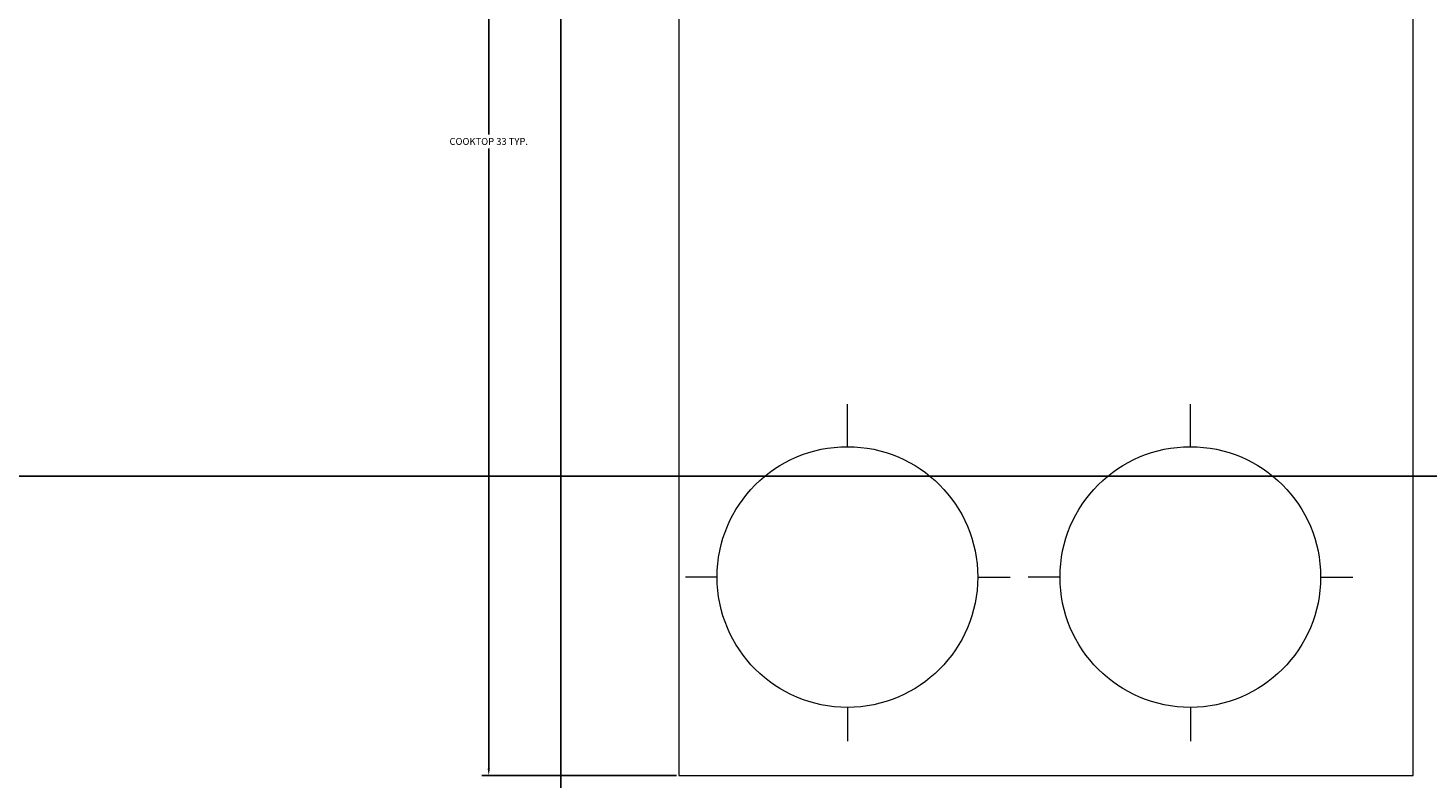
# Model space of a CAD drawing. Units: inches. Extents: x 1998 to 2588, y 1139 to 1977.
# Tile 22 of 134: x 2184 to 2220, y 1629 to 1648. Entities that reach past the tile are written whole.
import ezdxf

# ---------------------------------------------------------------- set-up
doc = ezdxf.new("R2010")
doc.units = ezdxf.units.IN
for name, color, linetype, lineweight in [('A-ANNO-DIMS', 2, 'Continuous', 18), ('A-EQPM', 21, 'Continuous', 18), ('A-FLOR-CASE', 32, 'Continuous', 25)]:
    doc.layers.add(name, color=color, linetype=linetype, lineweight=lineweight)
doc.styles.get("Standard").update_dxf_attribs({"font": 'arial.ttf'})
doc.dimstyles.get("Standard").update_dxf_attribs({"dimtxt": 0.18, "dimasz": 0.18, "dimexe": 0.18, "dimexo": 0.0625, "dimgap": 0.09, "dimtad": 0, "dimtih": 1, "dimtoh": 1, "dimdec": 4, "dimzin": 0, "dimdsep": 46, "dimtxsty": 'Standard', "dimcen": 0.09, "dimadec": 0, "dimazin": 0, "dimtfac": 1, "dimtdec": 4, "dimtofl": 0, "dimtmove": 0, "dimatfit": 3, "dimfxl": 1, "dimtolj": 1, "dimtzin": 0, "dimarcsym": 0})

# ---------------------------------------------------------------- blocks, each defined once
blk = doc.blocks.new('COOKTOP-FOUR-BURNER')
for p, q in [((13.348, 30.321), (13.348, 31.429)), ((16.748, 26.92), (17.591, 26.92)), ((4.474, 23.439), (4.474, 22.555)), ((13.348, 23.519), (13.348, 22.636)), ((4.399, 8.578), (4.399, 9.686)), ((13.348, 8.578), (13.348, 9.686)), ((0.999, 5.177), (0.172, 5.177)), ((7.8, 5.177), (8.642, 5.177)), ((9.947, 5.177), (9.12, 5.177)), ((16.748, 5.177), (17.591, 5.177)), ((4.399, 1.776), (4.399, 0.893)), ((13.348, 1.776), (13.348, 0.893))]:
    blk.add_line(p, q)
blk.add_lwpolyline([(19.165, 33.081), (0, 33.081), (0, 0), (19.165, 0)], close=True)
for centre in [(4.474, 26.84), (13.348, 26.92), (4.399, 5.177), (13.348, 5.177)]:
    blk.add_circle(centre, 3.401)
blk = doc.blocks.new('*D21')
at = {"layer": 'A-ANNO-DIMS', "color": 0, "lineweight": -2, "transparency": 16777216}
for p, q in [((2200.466, 1662.007), (2195.387, 1662.007)), ((2195.567, 1661.827), (2195.567, 1645.65)), ((2195.567, 1629.106), (2195.567, 1645.283)), ((2200.466, 1628.926), (2195.387, 1628.926))]:
    blk.add_line(p, q, dxfattribs=at)
at = {"layer": 'A-ANNO-DIMS', "color": 0, "transparency": 16777216}
for points in [[(2195.537, 1661.827), (2195.597, 1661.827), (2195.567, 1662.007)], [(2195.537, 1629.106), (2195.597, 1629.106), (2195.567, 1628.926)]]:
    blk.add_solid(points, dxfattribs=at)
at = {"layer": 'Defpoints', "color": 0, "transparency": 16777216}
for p in [(2195.567, 1662.007), (2200.529, 1662.007), (2200.529, 1628.926)]:
    blk.add_point(p, dxfattribs=at)
at = {"layer": 'A-ANNO-DIMS', "color": 0, "transparency": 16777216, "insert": (2195.567, 1645.467), "char_height": 0.18, "attachment_point": 5}
blk.add_mtext('\\A1;COOKTOP 33 TYP.', dxfattribs=at)
blk = doc.blocks.new('*D30')
at = {"layer": 'A-ANNO-DIMS', "color": 0, "lineweight": -2, "transparency": 16777216}
for p, q in [((2407.91, 1636.732), (1997.843, 1636.732)), ((1998.023, 1636.552), (1998.023, 1615.913)), ((1998.023, 1594.912), (1998.023, 1615.552)), ((2407.91, 1594.732), (1997.843, 1594.732))]:
    blk.add_line(p, q, dxfattribs=at)
at = {"layer": 'A-ANNO-DIMS', "color": 0, "transparency": 16777216}
for points in [[(1997.993, 1636.552), (1998.053, 1636.552), (1998.023, 1636.732)], [(1997.993, 1594.912), (1998.053, 1594.912), (1998.023, 1594.732)]]:
    blk.add_solid(points, dxfattribs=at)
at = {"layer": 'Defpoints', "color": 0, "transparency": 16777216}
for p in [(1998.023, 1636.732), (2407.973, 1636.732), (2407.973, 1594.732)]:
    blk.add_point(p, dxfattribs=at)
at = {"layer": 'A-ANNO-DIMS', "color": 0, "transparency": 16777216, "insert": (1998.023, 1615.732), "char_height": 0.18, "attachment_point": 5}
blk.add_mtext('\\A1;42', dxfattribs=at)
blk = doc.blocks.new('*D37')
at = {"layer": 'A-ANNO-DIMS', "color": 0, "lineweight": -2, "transparency": 16777216}
for p, q in [((2148.455, 1612.795), (2148.455, 1977.362)), ((2197.45, 1612.795), (2197.45, 1977.362)), ((2148.635, 1977.182), (2172.73, 1977.182)), ((2197.27, 1977.182), (2173.175, 1977.182))]:
    blk.add_line(p, q, dxfattribs=at)
at = {"layer": 'A-ANNO-DIMS', "color": 0, "transparency": 16777216}
for points in [[(2148.635, 1977.212), (2148.635, 1977.152), (2148.455, 1977.182)], [(2197.27, 1977.212), (2197.27, 1977.152), (2197.45, 1977.182)]]:
    blk.add_solid(points, dxfattribs=at)
at = {"layer": 'Defpoints', "color": 0, "transparency": 16777216}
for p in [(2197.45, 1977.182), (2148.455, 1612.732), (2197.45, 1612.732)]:
    blk.add_point(p, dxfattribs=at)
at = {"layer": 'A-ANNO-DIMS', "color": 0, "transparency": 16777216, "insert": (2172.952, 1977.182), "char_height": 0.18, "attachment_point": 5}
blk.add_mtext('\\A1;49', dxfattribs=at)
blk = doc.blocks.new('*D38')
at = {"layer": 'A-ANNO-DIMS', "color": 0, "lineweight": -2, "transparency": 16777216}
for p, q in [((2197.387, 1663.247), (1997.843, 1663.247)), ((1998.023, 1663.067), (1998.023, 1638.171)), ((1998.023, 1612.912), (1998.023, 1637.808)), ((2197.387, 1612.732), (1997.843, 1612.732))]:
    blk.add_line(p, q, dxfattribs=at)
at = {"layer": 'A-ANNO-DIMS', "color": 0, "transparency": 16777216}
for points in [[(1997.993, 1663.067), (1998.053, 1663.067), (1998.023, 1663.247)], [(1997.993, 1612.912), (1998.053, 1612.912), (1998.023, 1612.732)]]:
    blk.add_solid(points, dxfattribs=at)
at = {"layer": 'Defpoints', "color": 0, "transparency": 16777216}
for p in [(1998.023, 1663.247), (2197.45, 1663.247), (2197.45, 1612.732)]:
    blk.add_point(p, dxfattribs=at)
at = {"layer": 'A-ANNO-DIMS', "color": 0, "transparency": 16777216, "insert": (1998.023, 1637.99), "char_height": 0.18, "attachment_point": 5}
blk.add_mtext('\\A1;50.51', dxfattribs=at)

msp = doc.modelspace()

# ---------------------------------------------------------------- linework, layer by layer
at = {"layer": 'A-FLOR-CASE'}
msp.add_line((2197.4499, 1612.7324), (2197.4499, 1663.2466), dxfattribs=at)

# ---------------------------------------------------------------- block references
at = {"layer": 'A-EQPM'}
msp.add_blockref('COOKTOP-FOUR-BURNER', (2200.529, 1628.926), dxfattribs=at)

# ---------------------------------------------------------------- dimensions: what is measured, and where the dimension line sits
at = {"layer": 'A-ANNO-DIMS'}
dim = msp.add_linear_dim(base=(2197.4499, 1977.1824), p1=(2148.4548, 1612.7324), p2=(2197.4499, 1612.7324), dimstyle='Standard', override={"dimdec": 0, "dimlfac": 1, "dimrnd": 0, "dimzin": 0, "dimdsep": 46, "dimlunit": 2}, dxfattribs=at)
dim.commit()
dim.dimension.update_dxf_attribs({"geometry": '*D37', "text_midpoint": (2172.9524, 1977.1824)})
for base, p1, p2, override, picture, middle in [((1998.0229, 1663.2466), (2197.4499, 1612.7324), (2197.4499, 1663.2466), {"dimdec": 2, "dimlfac": 1, "dimrnd": 0, "dimzin": 0, "dimdsep": 46, "dimlunit": 2}, '*D38', (1998.0229, 1637.9895)), ((1998.0229, 1636.7324), (2407.9729, 1594.7324), (2407.9729, 1636.7324), {"dimdec": 0, "dimlfac": 1, "dimrnd": 0, "dimzin": 0, "dimdsep": 46, "dimlunit": 2}, '*D30', (1998.0229, 1615.7324))]:
    dim = msp.add_linear_dim(base=base, p1=p1, p2=p2, angle=90, dimstyle='Standard', override=override, dxfattribs=at)
    dim.commit()
    dim.dimension.update_dxf_attribs({"geometry": picture, "text_midpoint": middle})
dim = msp.add_linear_dim(base=(2195.5666, 1662.0068), p1=(2200.5286, 1628.9263), p2=(2200.5286, 1662.0068), angle=90, text='COOKTOP <> TYP.', dimstyle='Standard', override={"dimdec": 0, "dimlfac": 1, "dimrnd": 0, "dimzin": 0, "dimdsep": 46, "dimlunit": 2}, dxfattribs=at)
dim.commit()
dim.dimension.update_dxf_attribs({"geometry": '*D21', "text_midpoint": (2195.5666, 1645.4665)})

doc.saveas('drawing.dxf')
